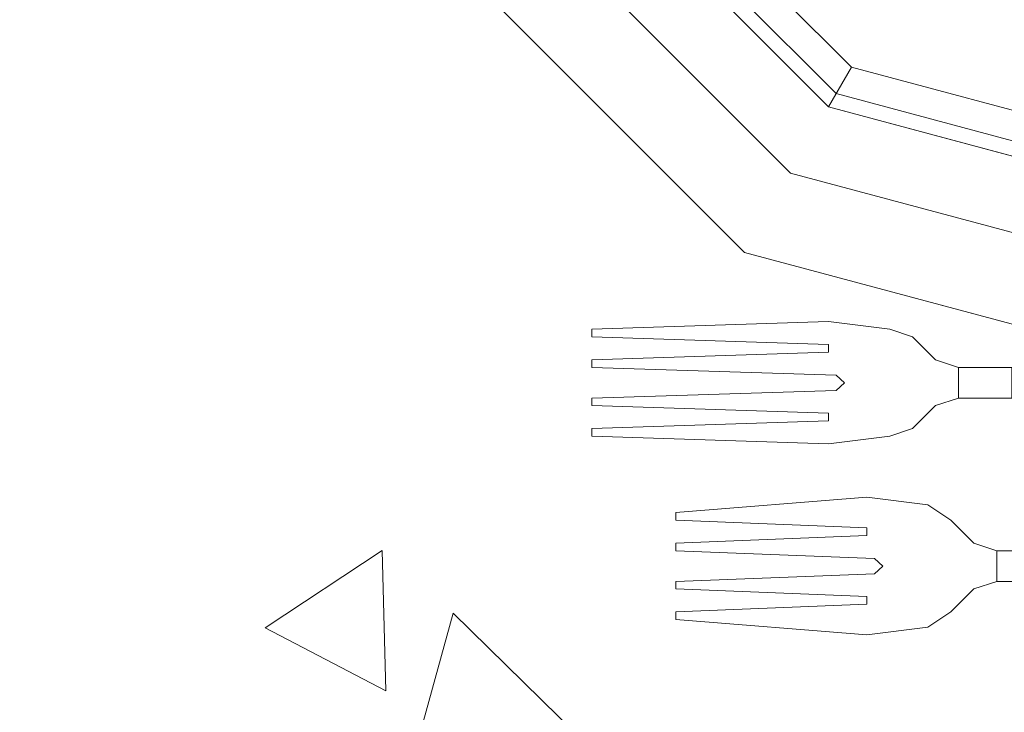
# Model space of a CAD drawing. Units: inches. Extents: x 375 to 1122, y 27 to 1069.
# Tile 136 of 155: x 731.16 to 739.094, y 886.613 to 892.194. Entities that reach past the tile are written whole.
import ezdxf

# ---------------------------------------------------------------- set-up
doc = ezdxf.new("R2010")
doc.units = ezdxf.units.IN
doc.layers.add('A-ANNO-DIMS', color=2, linetype='Continuous', lineweight=18)
doc.layers.add('Furniture', color=30, linetype='Continuous', lineweight=18)
doc.styles.get("Standard").update_dxf_attribs({"font": 'arial.ttf'})
doc.dimstyles.new('ISO-25', dxfattribs={"dimtxt": 12, "dimasz": 2.5, "dimexe": 1.5, "dimexo": 1.5, "dimtad": 1, "dimdec": 1, "dimlunit": 3, "dimtxsty": 'Standard', "dimblk": 'ARCHTICK', "dimcen": 2.5, "dimadec": 0, "dimazin": 0, "dimtfac": 1, "dimtdec": 1, "dimtmove": 0, "dimatfit": 3, "dimfxl": 1.5, "dimfxlon": 1, "dimarcsym": 0})

# ---------------------------------------------------------------- blocks, each defined once
blk = doc.blocks.new('A$C403C54AD')
for p, q in [((1.27568, 1.33837, -0.03581), (1.2726, 1.34298, -0.03534)), ((1.27568, 1.33837, -0.03888), (1.2726, 1.34298, -0.03842)), ((1.2372, 1.33067, -0.03581), (1.23566, 1.33529, -0.03534)), ((1.2372, 1.33067, -0.03888), (1.23566, 1.33529, -0.03842)), ((1.27287, 1.24271, -0.0006), (1.30033, 1.27073, -0.0006)), ((1.31179, 1.23198, -0.0006), (1.27287, 1.24271, -0.0006)), ((1.26024, 1.22842, -0.0006), (1.28849, 1.22914, -0.0006)), ((1.27579, 1.2048, -0.0006), (1.26024, 1.22842, -0.0006)), ((1.28849, 1.22914, -0.0006), (1.27579, 1.2048, -0.0006))]:
    blk.add_line(p, q)
at = {"linetype": 'ByBlock'}
for points, invisible_edges in [([(1.16818, 1.3199, -0.02965), (1.0802, 1.37069, -0.02965), (1.0802, 1.37069, -0.02965), (1.18179, 1.37069, -0.02965)], 5), ([(1.131, 1.28271, -0.02965), (1.0802, 1.37069, -0.02965), (1.0802, 1.37069, -0.02965), (1.16818, 1.3199, -0.02965)], 5), ([(1.18418, 1.31066, -0.02349), (1.16818, 1.3199, -0.02965), (1.18179, 1.37069, -0.02965), (1.20026, 1.37069, -0.02349)], 5), ([(1.17085, 1.31836, -0.03734), (1.20017, 1.30143, -0.02811), (1.21873, 1.37069, -0.02811), (1.18487, 1.37069, -0.03734)], 5), ([(1.20017, 1.30143, -0.02349), (1.18418, 1.31066, -0.02349), (1.20026, 1.37069, -0.02349), (1.21873, 1.37069, -0.02349)], 5), ([(1.12792, 1.28804, -0.04658), (1.13254, 1.28005, -0.03734), (1.17085, 1.31836, -0.03734), (1.16285, 1.32297, -0.04658)], 1), ([(1.14023, 1.26672, -0.02349), (1.131, 1.28271, -0.02965), (1.16818, 1.3199, -0.02965), (1.18418, 1.31066, -0.02349)], 5), ([(1.13254, 1.28005, -0.03734), (1.14947, 1.25072, -0.02811), (1.20017, 1.30143, -0.02811), (1.17085, 1.31836, -0.03734)], 5), ([(1.14947, 1.25072, -0.02349), (1.14023, 1.26672, -0.02349), (1.18418, 1.31066, -0.02349), (1.20017, 1.30143, -0.02349)], 5)]:
    blk.add_3dface(points, dxfattribs=dict(at, invisible_edges=invisible_edges))
for points in [[(1.16285, 1.32297, -0.04658), (1.17085, 1.31836, -0.03734), (1.18487, 1.37069, -0.03734), (1.17563, 1.37069, -0.04658)], [(1.20017, 1.30143, -0.02811), (1.20017, 1.30143, -0.02349), (1.21873, 1.37069, -0.02349), (1.21873, 1.37069, -0.02811)], [(1.14947, 1.25072, -0.02811), (1.14947, 1.25072, -0.02349), (1.20017, 1.30143, -0.02349), (1.20017, 1.30143, -0.02811)]]:
    blk.add_3dface(points, dxfattribs=at)
for points in [[(1.26645, 1.36299, -0.02863), (1.26029, 1.36299, -0.02863), (1.26029, 1.35222, -0.03071), (1.26645, 1.35222, -0.03071)], [(1.26645, 1.36299, -0.03122), (1.26029, 1.36299, -0.03122), (1.26029, 1.35222, -0.0333), (1.26645, 1.35222, -0.0333)], [(1.22951, 1.3553, -0.02863), (1.22335, 1.3553, -0.02863), (1.22335, 1.34452, -0.03071), (1.22951, 1.34452, -0.03071)], [(1.22951, 1.3553, -0.03122), (1.22335, 1.3553, -0.03122), (1.22335, 1.34452, -0.0333), (1.22951, 1.34452, -0.0333)], [(1.25721, 1.34606, -0.0341), (1.25721, 1.34606, -0.03718), (1.25413, 1.34298, -0.03842), (1.25413, 1.34298, -0.03534)], [(1.26953, 1.34606, -0.03718), (1.26953, 1.34606, -0.0341), (1.2726, 1.34298, -0.03534), (1.2726, 1.34298, -0.03842)], [(1.22027, 1.33837, -0.0341), (1.22027, 1.33837, -0.03718), (1.21719, 1.33529, -0.03842), (1.21719, 1.33529, -0.03534)], [(1.23258, 1.33837, -0.03718), (1.23258, 1.33837, -0.0341), (1.23566, 1.33529, -0.03534), (1.23566, 1.33529, -0.03842)], [(1.26337, 1.32925, -0.03868), (1.26337, 1.32925, -0.0356), (1.26183, 1.32759, -0.03545), (1.26183, 1.32759, -0.03853)], [(1.26491, 1.32759, -0.03545), (1.26491, 1.32759, -0.03853), (1.26337, 1.32925, -0.03868), (1.26337, 1.32925, -0.0356)], [(1.26029, 1.28757, -0.03119), (1.26029, 1.28757, -0.02811), (1.26183, 1.32759, -0.03545), (1.26183, 1.32759, -0.03853)], [(1.26491, 1.32759, -0.03853), (1.26491, 1.32759, -0.03545), (1.26645, 1.28757, -0.02811), (1.26645, 1.28757, -0.03119)], [(1.24952, 1.32605, -0.03829), (1.24952, 1.32605, -0.03521), (1.25259, 1.28757, -0.02811), (1.25259, 1.28757, -0.03119)], [(1.25413, 1.28757, -0.02811), (1.25413, 1.28757, -0.03119), (1.25567, 1.32605, -0.03829), (1.25567, 1.32605, -0.03521)], [(1.25721, 1.32605, -0.03829), (1.25721, 1.32605, -0.03521), (1.25567, 1.32605, -0.03521), (1.25567, 1.32605, -0.03829)], [(1.25721, 1.32605, -0.03829), (1.25721, 1.32605, -0.03521), (1.25875, 1.28757, -0.02811), (1.25875, 1.28757, -0.03119)], [(1.26799, 1.28757, -0.02811), (1.26799, 1.28757, -0.03119), (1.26953, 1.32605, -0.03829), (1.26953, 1.32605, -0.03521)], [(1.27106, 1.32605, -0.03521), (1.27106, 1.32605, -0.03829), (1.26953, 1.32605, -0.03829), (1.26953, 1.32605, -0.03521)], [(1.27106, 1.32605, -0.03521), (1.27106, 1.32605, -0.03829), (1.2726, 1.28757, -0.03119), (1.2726, 1.28757, -0.02811)], [(1.27414, 1.28757, -0.02811), (1.27414, 1.28757, -0.03119), (1.27722, 1.32605, -0.03829), (1.27722, 1.32605, -0.03521)], [(1.22643, 1.32156, -0.03868), (1.22643, 1.32156, -0.0356), (1.22489, 1.3199, -0.03545), (1.22489, 1.3199, -0.03853)], [(1.22797, 1.3199, -0.03545), (1.22797, 1.3199, -0.03853), (1.22643, 1.32156, -0.03868), (1.22643, 1.32156, -0.0356)], [(1.22335, 1.27064, -0.03119), (1.22335, 1.27064, -0.02811), (1.22489, 1.3199, -0.03545), (1.22489, 1.3199, -0.03853)], [(1.22797, 1.3199, -0.03853), (1.22797, 1.3199, -0.03545), (1.22951, 1.27064, -0.02811), (1.22951, 1.27064, -0.03119)], [(1.21411, 1.31836, -0.03829), (1.21411, 1.31836, -0.03521), (1.21565, 1.27064, -0.02811), (1.21565, 1.27064, -0.03119)], [(1.21719, 1.27064, -0.02811), (1.21719, 1.27064, -0.03119), (1.21873, 1.31836, -0.03829), (1.21873, 1.31836, -0.03521)], [(1.22027, 1.31836, -0.03829), (1.22027, 1.31836, -0.03521), (1.21873, 1.31836, -0.03521), (1.21873, 1.31836, -0.03829)], [(1.22027, 1.31836, -0.03829), (1.22027, 1.31836, -0.03521), (1.22181, 1.27064, -0.02811), (1.22181, 1.27064, -0.03119)], [(1.23105, 1.27064, -0.02811), (1.23105, 1.27064, -0.03119), (1.23258, 1.31836, -0.03829), (1.23258, 1.31836, -0.03521)], [(1.23412, 1.31836, -0.03521), (1.23412, 1.31836, -0.03829), (1.23258, 1.31836, -0.03829), (1.23258, 1.31836, -0.03521)], [(1.23412, 1.31836, -0.03521), (1.23412, 1.31836, -0.03829), (1.23566, 1.27064, -0.03119), (1.23566, 1.27064, -0.02811)], [(1.2372, 1.27064, -0.02811), (1.2372, 1.27064, -0.03119), (1.23874, 1.31836, -0.03829), (1.23874, 1.31836, -0.03521)], [(1.25259, 1.28757, -0.03119), (1.25259, 1.28757, -0.02811), (1.25413, 1.28757, -0.02811), (1.25413, 1.28757, -0.03119)], [(1.25875, 1.28757, -0.03119), (1.25875, 1.28757, -0.02811), (1.26029, 1.28757, -0.02811), (1.26029, 1.28757, -0.03119)], [(1.26645, 1.28757, -0.03119), (1.26645, 1.28757, -0.02811), (1.26799, 1.28757, -0.02811), (1.26799, 1.28757, -0.03119)], [(1.2726, 1.28757, -0.03119), (1.2726, 1.28757, -0.02811), (1.27414, 1.28757, -0.02811), (1.27414, 1.28757, -0.03119)], [(1.21565, 1.27064, -0.03119), (1.21565, 1.27064, -0.02811), (1.21719, 1.27064, -0.02811), (1.21719, 1.27064, -0.03119)], [(1.22181, 1.27064, -0.03119), (1.22181, 1.27064, -0.02811), (1.22335, 1.27064, -0.02811), (1.22335, 1.27064, -0.03119)], [(1.22951, 1.27064, -0.03119), (1.22951, 1.27064, -0.02811), (1.23105, 1.27064, -0.02811), (1.23105, 1.27064, -0.03119)], [(1.23566, 1.27064, -0.03119), (1.23566, 1.27064, -0.02811), (1.2372, 1.27064, -0.02811), (1.2372, 1.27064, -0.03119)]]:
    blk.add_3dface(points)
for points, invisible_edges in [([(1.26029, 1.36299, -0.03122), (1.26029, 1.36299, -0.02863), (1.26029, 1.35222, -0.03071), (1.26029, 1.35222, -0.0333)], 5), ([(1.26645, 1.35222, -0.0333), (1.26645, 1.35222, -0.03071), (1.26645, 1.36299, -0.02863), (1.26645, 1.36299, -0.03122)], 5), ([(1.22335, 1.3553, -0.03122), (1.22335, 1.3553, -0.02863), (1.22335, 1.34452, -0.03071), (1.22335, 1.34452, -0.0333)], 5), ([(1.22951, 1.34452, -0.0333), (1.22951, 1.34452, -0.03071), (1.22951, 1.3553, -0.02863), (1.22951, 1.3553, -0.03122)], 5), ([(1.26029, 1.35222, -0.03071), (1.26645, 1.35222, -0.03071), (1.26799, 1.3476, -0.03306), (1.25875, 1.3476, -0.03306)], 4), ([(1.26029, 1.35222, -0.0333), (1.26645, 1.35222, -0.0333), (1.26799, 1.3476, -0.03584), (1.25875, 1.3476, -0.03584)], 4), ([(1.26029, 1.35222, -0.03071), (1.26029, 1.35222, -0.0333), (1.25875, 1.3476, -0.03584), (1.25875, 1.3476, -0.03306)], 5), ([(1.26645, 1.35222, -0.0333), (1.26645, 1.35222, -0.03071), (1.26799, 1.3476, -0.03306), (1.26799, 1.3476, -0.03584)], 5), ([(1.26799, 1.3476, -0.03306), (1.25875, 1.3476, -0.03306), (1.25721, 1.34606, -0.0341), (1.26953, 1.34606, -0.0341)], 5), ([(1.26799, 1.3476, -0.03584), (1.25875, 1.3476, -0.03584), (1.25721, 1.34606, -0.03718), (1.26953, 1.34606, -0.03718)], 5), ([(1.25875, 1.3476, -0.03584), (1.25875, 1.3476, -0.03306), (1.25721, 1.34606, -0.0341), (1.25721, 1.34606, -0.03718)], 1), ([(1.26799, 1.3476, -0.03306), (1.26799, 1.3476, -0.03584), (1.26953, 1.34606, -0.03718), (1.26953, 1.34606, -0.0341)], 1), ([(1.26953, 1.34606, -0.03718), (1.25721, 1.34606, -0.03718), (1.25413, 1.34298, -0.03842), (1.2726, 1.34298, -0.03842)], 5), ([(1.26953, 1.34606, -0.0341), (1.25721, 1.34606, -0.0341), (1.25413, 1.34298, -0.03534), (1.2726, 1.34298, -0.03534)], 5), ([(1.22335, 1.34452, -0.03071), (1.22951, 1.34452, -0.03071), (1.23105, 1.33991, -0.03306), (1.22181, 1.33991, -0.03306)], 4), ([(1.22335, 1.34452, -0.03071), (1.22335, 1.34452, -0.0333), (1.22181, 1.33991, -0.03584), (1.22181, 1.33991, -0.03306)], 5), ([(1.22335, 1.34452, -0.0333), (1.22951, 1.34452, -0.0333), (1.23105, 1.33991, -0.03584), (1.22181, 1.33991, -0.03584)], 4), ([(1.22951, 1.34452, -0.0333), (1.22951, 1.34452, -0.03071), (1.23105, 1.33991, -0.03306), (1.23105, 1.33991, -0.03584)], 5), ([(1.25413, 1.34298, -0.03534), (1.2726, 1.34298, -0.03534), (1.27568, 1.33837, -0.03581), (1.25105, 1.33837, -0.03581)], 5), ([(1.25413, 1.34298, -0.03842), (1.2726, 1.34298, -0.03842), (1.27568, 1.33837, -0.03888), (1.25105, 1.33837, -0.03888)], 5), ([(1.25413, 1.34298, -0.03842), (1.25413, 1.34298, -0.03534), (1.25105, 1.33837, -0.03581), (1.25105, 1.33837, -0.03888)], 4), ([(1.2726, 1.34298, -0.03534), (1.2726, 1.34298, -0.03842), (1.27568, 1.33837, -0.03888), (1.27568, 1.33837, -0.03581)], 4), ([(1.23105, 1.33991, -0.03306), (1.22181, 1.33991, -0.03306), (1.22027, 1.33837, -0.0341), (1.23258, 1.33837, -0.0341)], 5), ([(1.23105, 1.33991, -0.03584), (1.22181, 1.33991, -0.03584), (1.22027, 1.33837, -0.03718), (1.23258, 1.33837, -0.03718)], 5), ([(1.22181, 1.33991, -0.03584), (1.22181, 1.33991, -0.03306), (1.22027, 1.33837, -0.0341), (1.22027, 1.33837, -0.03718)], 1), ([(1.23105, 1.33991, -0.03306), (1.23105, 1.33991, -0.03584), (1.23258, 1.33837, -0.03718), (1.23258, 1.33837, -0.0341)], 1), ([(1.23258, 1.33837, -0.03718), (1.22027, 1.33837, -0.03718), (1.21719, 1.33529, -0.03842), (1.23566, 1.33529, -0.03842)], 5), ([(1.23258, 1.33837, -0.0341), (1.22027, 1.33837, -0.0341), (1.21719, 1.33529, -0.03534), (1.23566, 1.33529, -0.03534)], 5), ([(1.25105, 1.33837, -0.03581), (1.25721, 1.32605, -0.03521), (1.25567, 1.32605, -0.03521), (1.24952, 1.32605, -0.03521)], 5), ([(1.25105, 1.33837, -0.03888), (1.25721, 1.32605, -0.03829), (1.25567, 1.32605, -0.03829), (1.24952, 1.32605, -0.03829)], 5), ([(1.25105, 1.33837, -0.03581), (1.25105, 1.33837, -0.03888), (1.24952, 1.32605, -0.03829), (1.24952, 1.32605, -0.03521)], 1), ([(1.25105, 1.33837, -0.03581), (1.26337, 1.32925, -0.0356), (1.26183, 1.32759, -0.03545), (1.25721, 1.32605, -0.03521)], 13), ([(1.25105, 1.33837, -0.03581), (1.26337, 1.32925, -0.0356), (1.27568, 1.33837, -0.03581), (1.25105, 1.33837, -0.03581)], 7), ([(1.25105, 1.33837, -0.03888), (1.26337, 1.32925, -0.03868), (1.26183, 1.32759, -0.03853), (1.25721, 1.32605, -0.03829)], 13), ([(1.25105, 1.33837, -0.03888), (1.26337, 1.32925, -0.03868), (1.27568, 1.33837, -0.03888), (1.25105, 1.33837, -0.03888)], 7), ([(1.27568, 1.33837, -0.03581), (1.26337, 1.32925, -0.0356), (1.26491, 1.32759, -0.03545), (1.26953, 1.32605, -0.03521)], 13), ([(1.27568, 1.33837, -0.03888), (1.26337, 1.32925, -0.03868), (1.26491, 1.32759, -0.03853), (1.26953, 1.32605, -0.03829)], 13), ([(1.27568, 1.33837, -0.03581), (1.26953, 1.32605, -0.03521), (1.27106, 1.32605, -0.03521), (1.27722, 1.32605, -0.03521)], 5), ([(1.27568, 1.33837, -0.03888), (1.26953, 1.32605, -0.03829), (1.27106, 1.32605, -0.03829), (1.27722, 1.32605, -0.03829)], 5), ([(1.27568, 1.33837, -0.03888), (1.27568, 1.33837, -0.03581), (1.27722, 1.32605, -0.03521), (1.27722, 1.32605, -0.03829)], 1), ([(1.21719, 1.33529, -0.03534), (1.23566, 1.33529, -0.03534), (1.2372, 1.33067, -0.03581), (1.21565, 1.33067, -0.03581)], 5), ([(1.21719, 1.33529, -0.03842), (1.23566, 1.33529, -0.03842), (1.2372, 1.33067, -0.03888), (1.21565, 1.33067, -0.03888)], 5), ([(1.21719, 1.33529, -0.03842), (1.21719, 1.33529, -0.03534), (1.21565, 1.33067, -0.03581), (1.21565, 1.33067, -0.03888)], 4), ([(1.23566, 1.33529, -0.03534), (1.23566, 1.33529, -0.03842), (1.2372, 1.33067, -0.03888), (1.2372, 1.33067, -0.03581)], 4), ([(1.21565, 1.33067, -0.03581), (1.22027, 1.31836, -0.03521), (1.21873, 1.31836, -0.03521), (1.21411, 1.31836, -0.03521)], 5), ([(1.21565, 1.33067, -0.03888), (1.22027, 1.31836, -0.03829), (1.21873, 1.31836, -0.03829), (1.21411, 1.31836, -0.03829)], 5), ([(1.21565, 1.33067, -0.03581), (1.21565, 1.33067, -0.03888), (1.21411, 1.31836, -0.03829), (1.21411, 1.31836, -0.03521)], 1), ([(1.21565, 1.33067, -0.03581), (1.22643, 1.32156, -0.0356), (1.22489, 1.3199, -0.03545), (1.22027, 1.31836, -0.03521)], 13), ([(1.21565, 1.33067, -0.03581), (1.22643, 1.32156, -0.0356), (1.2372, 1.33067, -0.03581), (1.21565, 1.33067, -0.03581)], 7), ([(1.21565, 1.33067, -0.03888), (1.22643, 1.32156, -0.03868), (1.2372, 1.33067, -0.03888), (1.21565, 1.33067, -0.03888)], 7), ([(1.21565, 1.33067, -0.03888), (1.22643, 1.32156, -0.03868), (1.22489, 1.3199, -0.03853), (1.22027, 1.31836, -0.03829)], 13), ([(1.2372, 1.33067, -0.03581), (1.22643, 1.32156, -0.0356), (1.22797, 1.3199, -0.03545), (1.23258, 1.31836, -0.03521)], 13), ([(1.2372, 1.33067, -0.03888), (1.22643, 1.32156, -0.03868), (1.22797, 1.3199, -0.03853), (1.23258, 1.31836, -0.03829)], 13), ([(1.2372, 1.33067, -0.03581), (1.23258, 1.31836, -0.03521), (1.23412, 1.31836, -0.03521), (1.23874, 1.31836, -0.03521)], 5), ([(1.2372, 1.33067, -0.03888), (1.23258, 1.31836, -0.03829), (1.23412, 1.31836, -0.03829), (1.23874, 1.31836, -0.03829)], 5), ([(1.2372, 1.33067, -0.03888), (1.2372, 1.33067, -0.03581), (1.23874, 1.31836, -0.03521), (1.23874, 1.31836, -0.03829)], 1), ([(1.25721, 1.32605, -0.03521), (1.26183, 1.32759, -0.03545), (1.26029, 1.28757, -0.02811), (1.25875, 1.28757, -0.02811)], 1), ([(1.25721, 1.32605, -0.03829), (1.26183, 1.32759, -0.03853), (1.26029, 1.28757, -0.03119), (1.25875, 1.28757, -0.03119)], 1), ([(1.26491, 1.32759, -0.03545), (1.26953, 1.32605, -0.03521), (1.26799, 1.28757, -0.02811), (1.26645, 1.28757, -0.02811)], 1), ([(1.26491, 1.32759, -0.03853), (1.26953, 1.32605, -0.03829), (1.26799, 1.28757, -0.03119), (1.26645, 1.28757, -0.03119)], 1), ([(1.25567, 1.32605, -0.03521), (1.24952, 1.32605, -0.03521), (1.25259, 1.28757, -0.02811), (1.25413, 1.28757, -0.02811)], 1), ([(1.25567, 1.32605, -0.03829), (1.24952, 1.32605, -0.03829), (1.25259, 1.28757, -0.03119), (1.25413, 1.28757, -0.03119)], 1), ([(1.27106, 1.32605, -0.03521), (1.27722, 1.32605, -0.03521), (1.27414, 1.28757, -0.02811), (1.2726, 1.28757, -0.02811)], 1), ([(1.27106, 1.32605, -0.03829), (1.27722, 1.32605, -0.03829), (1.27414, 1.28757, -0.03119), (1.2726, 1.28757, -0.03119)], 1), ([(1.22027, 1.31836, -0.03521), (1.22489, 1.3199, -0.03545), (1.22335, 1.27064, -0.02811), (1.22181, 1.27064, -0.02811)], 1), ([(1.22027, 1.31836, -0.03829), (1.22489, 1.3199, -0.03853), (1.22335, 1.27064, -0.03119), (1.22181, 1.27064, -0.03119)], 1), ([(1.22797, 1.3199, -0.03545), (1.23258, 1.31836, -0.03521), (1.23105, 1.27064, -0.02811), (1.22951, 1.27064, -0.02811)], 1), ([(1.22797, 1.3199, -0.03853), (1.23258, 1.31836, -0.03829), (1.23105, 1.27064, -0.03119), (1.22951, 1.27064, -0.03119)], 1), ([(1.21873, 1.31836, -0.03521), (1.21411, 1.31836, -0.03521), (1.21565, 1.27064, -0.02811), (1.21719, 1.27064, -0.02811)], 1), ([(1.21873, 1.31836, -0.03829), (1.21411, 1.31836, -0.03829), (1.21565, 1.27064, -0.03119), (1.21719, 1.27064, -0.03119)], 1), ([(1.23412, 1.31836, -0.03521), (1.23874, 1.31836, -0.03521), (1.2372, 1.27064, -0.02811), (1.23566, 1.27064, -0.02811)], 1), ([(1.23412, 1.31836, -0.03829), (1.23874, 1.31836, -0.03829), (1.2372, 1.27064, -0.03119), (1.23566, 1.27064, -0.03119)], 1)]:
    blk.add_3dface(points, dxfattribs=dict(invisible_edges=invisible_edges))
blk = doc.blocks.new('_ArchTick')
at = {"color": 0, "linetype": 'ByBlock', "const_width": 0.15}
blk.add_lwpolyline([(-0.5, -0.5), (0.5, 0.5)], dxfattribs=at)
blk = doc.blocks.new('*D88')
at = {"layer": 'A-ANNO-DIMS', "color": 0, "lineweight": -2, "transparency": 16777216}
for p, q in [((731.0073, 1052.5277), (731.0073, 1055.5277)), ((854.0073, 1052.5277), (854.0073, 1055.5277)), ((731.0073, 1054.0277), (854.0073, 1054.0277))]:
    blk.add_line(p, q, dxfattribs=at)
at = {"layer": 'Defpoints', "color": 0, "transparency": 16777216}
for p in [(854.0073, 1054.0277), (731.0073, 502.5277), (854.0073, 502.5277)]:
    blk.add_point(p, dxfattribs=at)
at = {"layer": 'A-ANNO-DIMS', "color": 0, "lineweight": -2, "transparency": 16777216, "xscale": 2.5, "yscale": 2.5, "zscale": 2.5, "rotation": 180}
blk.add_blockref('_ArchTick', (731.0073, 1054.0277), dxfattribs=at)
at = {"layer": 'A-ANNO-DIMS', "color": 0, "lineweight": -2, "transparency": 16777216, "xscale": 2.5, "yscale": 2.5, "zscale": 2.5}
blk.add_blockref('_ArchTick', (854.0073, 1054.0277), dxfattribs=at)
at = {"layer": 'A-ANNO-DIMS', "color": 0, "transparency": 16777216, "insert": (792.5073, 1060.7837), "char_height": 12, "attachment_point": 5}
blk.add_mtext('10\'-3"', dxfattribs=at)
blk = doc.blocks.new('*D91')
at = {"layer": 'A-ANNO-DIMS', "color": 0, "lineweight": -2, "transparency": 16777216}
for p, q in [((728.0073, 1052.5277), (728.0073, 1055.5277)), ((788.0073, 1052.5277), (788.0073, 1055.5277)), ((728.0073, 1054.0277), (788.0073, 1054.0277))]:
    blk.add_line(p, q, dxfattribs=at)
at = {"layer": 'Defpoints', "color": 0, "transparency": 16777216}
for p in [(788.0073, 1054.0277), (728.0073, 774.0277), (788.0073, 774.0277)]:
    blk.add_point(p, dxfattribs=at)
at = {"layer": 'A-ANNO-DIMS', "color": 0, "lineweight": -2, "transparency": 16777216, "xscale": 2.5, "yscale": 2.5, "zscale": 2.5, "rotation": 180}
blk.add_blockref('_ArchTick', (728.0073, 1054.0277), dxfattribs=at)
at = {"layer": 'A-ANNO-DIMS', "color": 0, "lineweight": -2, "transparency": 16777216, "xscale": 2.5, "yscale": 2.5, "zscale": 2.5}
blk.add_blockref('_ArchTick', (788.0073, 1054.0277), dxfattribs=at)
at = {"layer": 'A-ANNO-DIMS', "color": 0, "transparency": 16777216, "insert": (758.0073, 1060.7796), "char_height": 12, "attachment_point": 5}
blk.add_mtext('5\'-0"', dxfattribs=at)

msp = doc.modelspace()

# ---------------------------------------------------------------- block references
at = {"layer": 'Furniture', "xscale": 39.9918517141215, "yscale": 39.9918517141215, "zscale": 39.9918517141215, "rotation": 270}
msp.add_blockref('A$C403C54AD', (684.9549, 938.3156, 0.024), dxfattribs=at)

# ---------------------------------------------------------------- dimensions: what is measured, and where the dimension line sits
at = {"layer": 'A-ANNO-DIMS'}
for base, p1, p2, picture, middle in [((788.0073, 1054.0277), (728.0073, 774.0277), (788.0073, 774.0277), '*D91', (758.0073, 1060.7796)), ((854.0073, 1054.0277), (731.0073, 502.5277), (854.0073, 502.5277), '*D88', (792.5073, 1060.7837))]:
    dim = msp.add_linear_dim(base=base, p1=p1, p2=p2, dimstyle='ISO-25', override={"dimdec": 1, "dimlfac": 1, "dimrnd": 0, "dimzin": 1, "dimdsep": 46, "dimlunit": 4, "dimfrac": 2}, dxfattribs=at)
    dim.commit()
    dim.dimension.update_dxf_attribs({"geometry": picture, "text_midpoint": middle})

doc.saveas('drawing.dxf')
